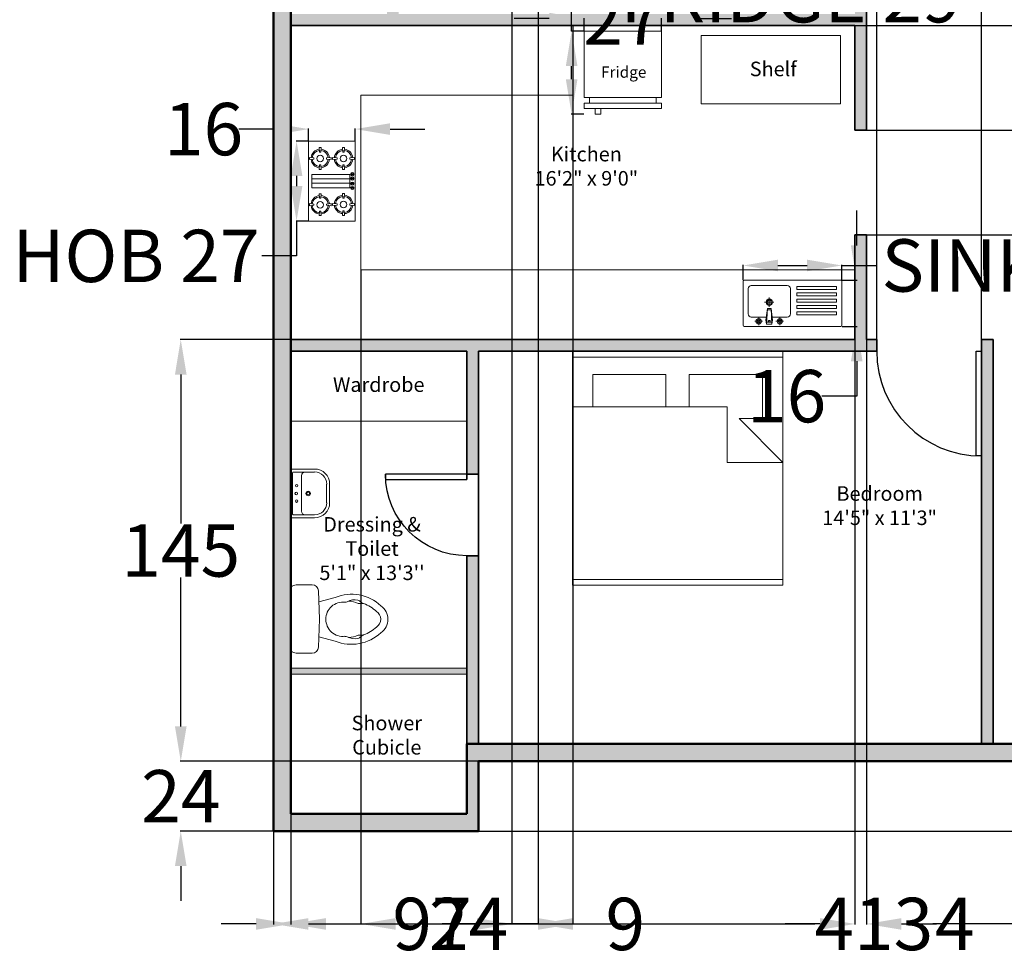
# Model space of a CAD drawing. Units: inches. Extents: x 2 to 695, y -374 to 352.
# Tile 1 of 6: x 59 to 398, y -374 to -51. Entities that reach past the tile are written whole.
import ezdxf

# ---------------------------------------------------------------- set-up
doc = ezdxf.new("R2010")
doc.units = ezdxf.units.IN
for name, color, linetype, lineweight in [('A-ANNO-DIMS', 2, 'Continuous', 18), ('A-ANNO-TEXT', 7, 'Continuous', 18), ('A-AREA-IDEN', 7, 'Continuous', 18), ('A-DOOR', 3, 'Continuous', 25), ('A-FLOR-FIXT', 9, 'Continuous', 18), ('A-WALL-PATT', 252, 'Continuous', 13), ('Furniture', 2, 'Continuous', 18), ('Inner Wall', 5, 'Continuous', 35), ('Kitchen', 6, 'Continuous', 18), ('Outer Wall', 1, 'Continuous', 50)]:
    doc.layers.add(name, color=color, linetype=linetype, lineweight=lineweight)
doc.styles.get("Standard").update_dxf_attribs({"font": 'arial.ttf'})
doc.dimstyles.get("Standard").update_dxf_attribs({"dimtxt": 18, "dimasz": 12, "dimexe": 0.18, "dimexo": 0.0625, "dimgap": 0.09, "dimtad": 0, "dimtih": 1, "dimtoh": 1, "dimdec": 0, "dimzin": 0, "dimdsep": 46, "dimlunit": 3, "dimtxsty": 'Standard', "dimcen": 0.09, "dimadec": 0, "dimazin": 0, "dimtfac": 1, "dimtdec": 0, "dimtofl": 0, "dimtmove": 0, "dimatfit": 3, "dimfxl": 1, "dimtolj": 1, "dimtzin": 0, "dimarcsym": 0})

# ---------------------------------------------------------------- blocks, each defined once
blk = doc.blocks.new('*U2')
for p, q in [((0, 0), (0, -4)), ((36, 0), (36, -4))]:
    blk.add_line(p, q)
blk.add_lwpolyline([(0, 0), (0, 36), (1.75, 36), (1.75, 0)], close=True)
blk.add_arc((0, 0), 36, 0, 90)
blk = doc.blocks.new('A$C7C492201')
for p, q in [((0, 10), (0, 426.6)), ((10, 436.6), (927.3, 436.6)), ((111.9, 388.7), (185, 388.7)), ((148.5, 425.2), (148.5, 352.2)), ((223.5, 415), (217, 376.2)), ((217, 376.2), (231.8, 268.5)), ((223.5, 415), (231.8, 268.5)), ((223.5, 415), (248.5, 415)), ((224.6, 395.4), (248.5, 395.4)), ((273.5, 415), (248.5, 415)), ((272.3, 395.4), (248.5, 395.4)), ((273.5, 415), (265.2, 268.5)), ((279.9, 376.2), (265.2, 268.5)), ((273.5, 415), (279.9, 376.2)), ((311.9, 388.7), (385, 388.7)), ((348.5, 425.2), (348.5, 352.2)), ((937.3, 10), (937.3, 426.6)), ((48.5, 318.8), (48.5, 78.8)), ((220.8, 348.8), (78.5, 348.8)), ((418.5, 348.8), (276.2, 348.8)), ((448.5, 318.8), (448.5, 78.8)), ((509.1, 328.4), (509.1, 298.4)), ((509.1, 328.4), (885, 328.4)), ((509.1, 298.4), (885, 298.4)), ((885, 328.4), (885, 298.4)), ((203.4, 207.7), (293.5, 207.7)), ((231.3, 278.6), (248.5, 278.6)), ((231.8, 268.5), (248.5, 268.5)), ((265.6, 278.6), (248.5, 278.6)), ((265.2, 268.5), (248.5, 268.5)), ((248.5, 252.8), (248.5, 162.6)), ((509.1, 268.4), (509.1, 238.4)), ((509.1, 268.4), (885, 268.4)), ((509.1, 238.4), (885, 238.4)), ((509.1, 208.4), (885, 208.4)), ((509.1, 208.4), (509.1, 178.4)), ((885, 268.4), (885, 238.4)), ((885, 208.4), (885, 178.4)), ((509.1, 178.4), (885, 178.4)), ((509.1, 148.4), (509.1, 118.4)), ((509.1, 148.4), (885, 148.4)), ((509.1, 118.4), (885, 118.4)), ((885, 148.4), (885, 118.4)), ((927.3, 0), (10, 0)), ((418.5, 48.8), (78.5, 48.8)), ((509.1, 88.4), (509.1, 58.4)), ((509.1, 88.4), (885, 88.4)), ((509.1, 58.4), (885, 58.4)), ((885, 88.4), (885, 58.4))]:
    blk.add_line(p, q)
for centre, radius in [((148.5, 388.7), 25), ((148.5, 388.7), 15), ((348.5, 388.7), 25), ((348.5, 388.7), 15), ((248.5, 207.7), 30), ((248.5, 207.7), 20)]:
    blk.add_circle(centre, radius)
for centre, radius, start, end in [((10, 426.6), 10, 90, 180), ((247.3, 388), 7.19, 80.52523, 279.47477), ((249.6, 388), 7.19, 260.52523, 99.47477), ((927.3, 426.6), 10, 0, 90), ((78.5, 318.8), 30, 90, 180), ((418.5, 318.8), 30, 0, 90), ((10, 10), 10, 180, 270), ((78.5, 78.8), 30, 180, 270), ((418.5, 78.8), 30, 270, 0), ((927.3, 10), 10, 270, 0)]:
    blk.add_arc(centre, radius, start, end)
blk = doc.blocks.new('A$C57CF26DA')
for p, q in [((0, 0), (0, 420)), ((720, 420), (0, 420)), ((166.9, 413), (146.9, 413)), ((146.9, 413), (151.9, 373)), ((151.9, 373), (161.9, 373)), ((161.9, 373), (166.9, 413)), ((300, 390.9), (300, 49.1)), ((300, 390.9), (420, 390.9)), ((340, 390.9), (340, 49.1)), ((380, 390.9), (380, 49.1)), ((420, 390.9), (420, 49.1)), ((583.6, 413), (563.6, 413)), ((563.6, 413), (568.6, 373)), ((568.6, 373), (578.6, 373)), ((578.6, 373), (583.6, 413)), ((720, 0), (720, 420)), ((98.9, 320), (58.9, 325)), ((58.9, 325), (58.9, 305)), ((58.9, 305), (98.9, 310)), ((98.9, 310), (98.9, 320)), ((254.8, 325), (214.8, 320)), ((214.8, 320), (214.8, 310)), ((214.8, 310), (254.8, 305)), ((254.8, 305), (254.8, 325)), ((515.6, 320), (475.6, 325)), ((475.6, 325), (475.6, 305)), ((475.6, 305), (515.6, 310)), ((515.6, 310), (515.6, 320)), ((671.6, 325), (631.6, 320)), ((631.6, 320), (631.6, 310)), ((631.6, 310), (671.6, 305)), ((671.6, 305), (671.6, 325)), ((151.9, 257), (146.9, 217)), ((146.9, 217), (166.9, 217)), ((166.9, 203), (146.9, 203)), ((146.9, 203), (151.9, 163)), ((161.9, 257), (151.9, 257)), ((166.9, 217), (161.9, 257)), ((161.9, 163), (166.9, 203)), ((581.1, 203), (561.1, 203)), ((561.1, 203), (566.1, 163)), ((568.6, 257), (563.6, 217)), ((563.6, 217), (583.6, 217)), ((578.6, 257), (568.6, 257)), ((576.1, 163), (581.1, 203)), ((583.6, 217), (578.6, 257)), ((98.9, 110), (58.9, 115)), ((58.9, 115), (58.9, 95)), ((58.9, 95), (98.9, 100)), ((98.9, 100), (98.9, 110)), ((151.9, 163), (161.9, 163)), ((254.8, 115), (214.8, 110)), ((214.8, 110), (214.8, 100)), ((214.8, 100), (254.8, 95)), ((254.8, 95), (254.8, 115)), ((513.1, 110), (473.1, 115)), ((473.1, 115), (473.1, 95)), ((473.1, 95), (513.1, 100)), ((513.1, 100), (513.1, 110)), ((566.1, 163), (576.1, 163)), ((669, 115), (629, 110)), ((629, 110), (629, 100)), ((629, 100), (669, 95)), ((669, 95), (669, 115)), ((151.9, 47), (146.9, 7)), ((146.9, 7), (166.9, 7)), ((161.9, 47), (151.9, 47)), ((166.9, 7), (161.9, 47)), ((301.5, 38.7), (294.7, 38.7)), ((294.7, 38.7), (294.7, 11.3)), ((294.7, 11.3), (301.5, 11.3)), ((420, 49.1), (300, 49.1)), ((301.5, 11.3), (301.5, 38.7)), ((340.5, 38.7), (333.7, 38.7)), ((333.7, 38.7), (333.7, 11.3)), ((333.7, 11.3), (340.5, 11.3)), ((340.5, 11.3), (340.5, 38.7)), ((379.7, 11.3), (379.7, 38.7)), ((379.7, 38.7), (386.5, 38.7)), ((386.5, 11.3), (379.7, 11.3)), ((386.5, 38.7), (386.5, 11.3)), ((418.7, 11.3), (418.7, 38.7)), ((418.7, 38.7), (425.5, 38.7)), ((425.5, 11.3), (418.7, 11.3)), ((425.5, 38.7), (425.5, 11.3)), ((566.1, 47), (561.1, 7)), ((561.1, 7), (581.1, 7)), ((576.1, 47), (566.1, 47)), ((581.1, 7), (576.1, 47)), ((720, 0), (0, 0))]:
    blk.add_line(p, q)
for centre in [(156.9, 315), (573.6, 315), (156.9, 105), (571.1, 105)]:
    blk.add_circle(centre, 30)
for centre, radius, start, end in [((156.9, 315), 83, 95.58493, 174.41507), ((156.9, 315), 73, 95.37384, 174.62616), ((156.9, 315), 73, 5.37384, 84.62616), ((156.9, 315), 83, 5.58493, 84.41507), ((573.6, 315), 83, 95.58493, 174.41507), ((573.6, 315), 73, 95.37384, 174.62616), ((573.6, 315), 73, 5.37384, 84.62616), ((573.6, 315), 83, 5.58493, 84.41507), ((156.9, 315), 83, 185.58493, 264.41507), ((156.9, 315), 73, 185.37384, 264.62616), ((156.9, 315), 73, 275.37384, 354.62616), ((156.9, 315), 83, 275.58493, 354.41507), ((573.6, 315), 83, 185.58493, 264.41507), ((573.6, 315), 73, 185.37384, 264.62616), ((573.6, 315), 73, 275.37384, 354.62616), ((573.6, 315), 83, 275.58493, 354.41507), ((156.9, 105), 83, 95.58493, 174.41507), ((156.9, 105), 73, 95.37384, 174.62616), ((156.9, 105), 73, 5.37384, 84.62616), ((156.9, 105), 83, 5.58493, 84.41507), ((571.1, 105), 83, 95.58493, 174.41507), ((571.1, 105), 73, 95.37384, 174.62616), ((571.1, 105), 73, 5.37384, 84.62616), ((571.1, 105), 83, 5.58493, 84.41507), ((156.9, 105), 83, 185.58493, 264.41507), ((156.9, 105), 73, 185.37384, 264.62616), ((156.9, 105), 73, 275.37384, 354.62616), ((156.9, 105), 83, 275.58493, 354.41507), ((571.1, 105), 83, 185.58493, 264.41507), ((571.1, 105), 73, 185.37384, 264.62616), ((571.1, 105), 73, 275.37384, 354.62616), ((571.1, 105), 83, 275.58493, 354.41507), ((298.1, 25), 13.7, 104.47751, 255.52249), ((298.1, 25), 13.7, 284.47751, 75.52249), ((337.1, 25), 13.7, 104.47751, 255.52249), ((337.1, 25), 13.7, 284.47751, 75.52249), ((383.1, 25), 13.7, 104.47751, 255.52249), ((383.1, 25), 13.7, 284.47751, 75.52249), ((422.1, 25), 13.7, 104.47751, 255.52249), ((422.1, 25), 13.7, 284.47751, 75.52249)]:
    blk.add_arc(centre, radius, start, end)
blk = doc.blocks.new('KING-00')
for p, q in [((-0.8967, -0.947), (-0.8967, 0.8818)), ((0.6019, 0.8818), (0.6019, -0.4644)), ((1.0337, -0.947), (1.0337, 0.8818)), ((0.6019, 0.704), (0.8813, 0.704)), ((0.8813, 0.069), (0.8813, 0.704)), ((0.6019, 0.069), (0.8813, 0.069)), ((0.8813, -0.1342), (0.6019, -0.1342)), ((0.8813, -0.7692), (0.8813, -0.1342)), ((0.1193, -0.4644), (0.1193, -0.947)), ((0.6019, -0.4644), (0.1193, -0.4644)), ((0.1193, -0.947), (0.5003, -0.566)), ((0.5003, -0.7692), (0.5003, -0.566)), ((0.5003, -0.7692), (0.8813, -0.7692))]:
    blk.add_line(p, q)
blk.add_lwpolyline([(-0.9475, -0.947), (-0.9475, 0.8818), (1.0845, 0.8818), (1.0845, -0.947)], close=True)
blk = doc.blocks.new('REFRI-00')
for points in [[(-0.35, 0.35), (-0.35, -0.25), (0.35, -0.25), (0.35, 0.35), (-0.35, 0.35)], [(-0.3, -0.3), (-0.3, -0.25)], [(0.3, -0.3), (0.3, -0.25)], [(-0.35, -0.3), (-0.35, -0.35), (0.35, -0.35), (0.35, -0.3), (-0.35, -0.3)], [(-0.25, -0.35), (-0.25, -0.4), (-0.2, -0.4), (-0.2, -0.35)]]:
    blk.add_lwpolyline(points)
blk = doc.blocks.new('A$C1308471B')
at = {"ltscale": 20}
for p, q in [((0, 0.4607), (0, 0.0186)), ((0.0354, 0.4793), (0.1495, 0.4793)), ((0.2013, 0.2397), (0.1923, 0.4384)), ((0.1957, 0.3639), (0.3109, 0.3953)), ((0.5021, 0.3528), (0.4724, 0.3528)), ((0.4982, 0.3575), (0.4822, 0.3709)), ((0.2013, 0.2397), (0.1923, 0.0409)), ((0.1959, 0.1193), (0.3109, 0.0879)), ((0.5021, 0.1304), (0.4724, 0.1304)), ((0.4982, 0.1257), (0.4822, 0.1123)), ((0.0354, 0), (0.1495, 0))]:
    blk.add_line(p, q, dxfattribs=at)
for centre, radius, start, end in [((0.006, 0.4607), 0.006, 136.52689, 180), ((0.0354, 0.4328), 0.0465, 90, 136.52689), ((0.1495, 0.4365), 0.0429, 2.57554, 90), ((0.4248, 0.1104), 0.3068, 47.41345, 111.79241), ((0.3654, 0.2416), 0.1206, 83.35226, 180), ((0.3823, 0.3868), 0.0255, 263.35226, 298.57415), ((0.4494, 0.2636), 0.1148, 79.39683, 118.57415), ((0.405, 0.2159), 0.153, 63.50202, 90.45216), ((0.4658, 0.3513), 0.0255, 50, 79.39683), ((0.5146, 0.377), 0.0255, 230, 251.38812), ((0.5021, 0.3273), 0.0255, 70.3751, 90), ((0.4248, 0.1104), 0.2558, 46.61198, 70.3751), ((0.5654, 0.2416), 0.065, 0, 57.29738), ((0.5654, 0.2416), 0.116, 0, 54.71147), ((0.3654, 0.2416), 0.1206, 180, 276.64774), ((0.5654, 0.2416), 0.065, 302.70262, 0), ((0.5654, 0.2416), 0.116, 305.28853, 0), ((0.4248, 0.3728), 0.3068, 248.20759, 312.58655), ((0.4248, 0.3728), 0.2558, 289.6249, 313.38802), ((0.3823, 0.0964), 0.0255, 61.42585, 96.64774), ((0.4494, 0.2196), 0.1148, 241.42585, 280.60317), ((0.405, 0.2673), 0.153, 269.54784, 296.49798), ((0.4658, 0.1319), 0.0255, 280.60317, 310), ((0.5146, 0.1062), 0.0255, 108.61188, 130), ((0.5021, 0.1559), 0.0255, 270, 289.6249), ((0.006, 0.0186), 0.006, 180, 223.47311), ((0.0354, 0.0465), 0.0465, 223.47311, 270), ((0.1495, 0.0429), 0.0429, 270, 357.42446)]:
    blk.add_arc(centre, radius, start, end, dxfattribs=at)
blk = doc.blocks.new('A$C57EA129C')
for p, q in [((0, 0.443), (0, 0.178)), ((0.016, 0.459), (0.563, 0.459)), ((0.036, 0.432), (0.036, 0.29)), ((0.045, 0.441), (0.535, 0.441)), ((0.544, 0.432), (0.544, 0.29)), ((0.579, 0.443), (0.579, 0.178)), ((0.036, 0.29), (0.036, 0.178)), ((0.08, 0.334), (0.499, 0.334)), ((0.544, 0.29), (0.544, 0.178)), ((0.178, 0.036), (0.401, 0.036)), ((0.178, 0), (0.401, 0))]:
    blk.add_line(p, q)
for centre, radius in [((0.198, 0.392), 0.0143), ((0.29, 0.396), 0.0156), ((0.381, 0.392), 0.0143), ((0.29, 0.255), 0.0267), ((0.29, 0.255), 0.0178)]:
    blk.add_circle(centre, radius)
for centre, radius, start, end in [((0.016, 0.443), 0.016, 90, 180), ((0.045, 0.432), 0.00891, 90, 180), ((0.535, 0.432), 0.00891, 0, 90), ((0.563, 0.443), 0.016, 0, 90), ((0.08, 0.29), 0.0445, 90, 180), ((0.499, 0.29), 0.0445, 0, 90), ((0.178, 0.178), 0.178, 180, 270), ((0.178, 0.178), 0.143, 180, 270), ((0.401, 0.178), 0.178, 270, 0), ((0.401, 0.178), 0.143, 270, 0)]:
    blk.add_arc(centre, radius, start, end)
blk = doc.blocks.new('*U3')
for p, q in [((0, 0), (0, -4)), ((28, 0), (28, -4))]:
    blk.add_line(p, q)
blk.add_lwpolyline([(0, 0), (0, 28), (1.75, 28), (1.75, 0)], close=True)
blk.add_arc((0, 0), 28, 0, 90)
blk = doc.blocks.new('*D22')
at = {"layer": 'A-ANNO-DIMS', "color": 0, "lineweight": -2, "transparency": 16777216}
for p, q in [((308.29, -140.37), (308.29, -135.15)), ((320.29, -135.33), (330.3, -135.33)), ((342.3, -140.37), (342.3, -135.15)), ((342.3, -135.33), (354.3, -135.33))]:
    blk.add_line(p, q, dxfattribs=at)
at = {"layer": 'A-ANNO-DIMS', "color": 0, "transparency": 16777216}
for points in [[(320.29, -133.33), (320.29, -137.33), (308.29, -135.33)], [(330.3, -133.33), (330.3, -137.33), (342.3, -135.33)]]:
    blk.add_solid(points, dxfattribs=at)
at = {"layer": 'Defpoints', "color": 0, "transparency": 16777216}
for p in [(342.3, -135.33), (308.29, -140.43), (342.3, -140.43)]:
    blk.add_point(p, dxfattribs=at)
at = {"layer": 'A-ANNO-DIMS', "color": 0, "transparency": 16777216, "insert": (400.04, -135.33), "char_height": 18, "attachment_point": 5}
blk.add_mtext('\\A1;SINK 34', dxfattribs=at)
blk = doc.blocks.new('*D23')
at = {"layer": 'A-ANNO-DIMS', "color": 0, "lineweight": -2, "transparency": 16777216}
for p, q in [((347.4, -128.43), (347.4, -116.43)), ((342.37, -140.43), (347.58, -140.43)), ((342.37, -156.27), (347.58, -156.27)), ((347.4, -168.27), (347.4, -180.27)), ((347.4, -180.27), (335.4, -180.27))]:
    blk.add_line(p, q, dxfattribs=at)
at = {"layer": 'A-ANNO-DIMS', "color": 0, "transparency": 16777216}
for points in [[(345.4, -128.43), (349.4, -128.43), (347.4, -140.43)], [(345.4, -168.27), (349.4, -168.27), (347.4, -156.27)]]:
    blk.add_solid(points, dxfattribs=at)
at = {"layer": 'Defpoints', "color": 0, "transparency": 16777216}
for p in [(342.3, -140.43), (342.3, -156.27), (347.4, -156.27)]:
    blk.add_point(p, dxfattribs=at)
at = {"layer": 'A-ANNO-DIMS', "color": 0, "transparency": 16777216, "insert": (323.28, -180.27), "char_height": 18, "attachment_point": 5}
blk.add_mtext('\\A1;16', dxfattribs=at)
blk = doc.blocks.new('*D24')
at = {"layer": 'A-ANNO-DIMS', "color": 0, "lineweight": -2, "transparency": 16777216}
for p, q in [((158.77, -92.56), (154.53, -92.56)), ((154.71, -104.56), (154.71, -108.04)), ((158.77, -120.04), (154.53, -120.04)), ((154.71, -120.04), (154.71, -132.04)), ((154.71, -132.04), (142.71, -132.04))]:
    blk.add_line(p, q, dxfattribs=at)
at = {"layer": 'A-ANNO-DIMS', "color": 0, "transparency": 16777216}
for points in [[(152.71, -104.56), (156.71, -104.56), (154.71, -92.56)], [(152.71, -108.04), (156.71, -108.04), (154.71, -120.04)]]:
    blk.add_solid(points, dxfattribs=at)
at = {"layer": 'Defpoints', "color": 0, "transparency": 16777216}
for p in [(158.84, -92.56), (154.71, -120.04), (158.84, -120.04)]:
    blk.add_point(p, dxfattribs=at)
at = {"layer": 'A-ANNO-DIMS', "color": 0, "transparency": 16777216, "insert": (99.48, -132.04), "char_height": 18, "attachment_point": 5}
blk.add_mtext('\\A1;HOB 27', dxfattribs=at)
blk = doc.blocks.new('*D25')
at = {"layer": 'A-ANNO-DIMS', "color": 0, "lineweight": -2, "transparency": 16777216}
for p, q in [((146.84, -88.44), (134.84, -88.44)), ((158.84, -92.5), (158.84, -88.26)), ((174.87, -92.5), (174.87, -88.26)), ((186.87, -88.44), (198.87, -88.44))]:
    blk.add_line(p, q, dxfattribs=at)
at = {"layer": 'A-ANNO-DIMS', "color": 0, "transparency": 16777216}
for points in [[(146.84, -86.44), (146.84, -90.44), (158.84, -88.44)], [(186.87, -86.44), (186.87, -90.44), (174.87, -88.44)]]:
    blk.add_solid(points, dxfattribs=at)
at = {"layer": 'Defpoints', "color": 0, "transparency": 16777216}
for p in [(158.84, -88.44), (158.84, -92.56), (174.87, -92.56)]:
    blk.add_point(p, dxfattribs=at)
at = {"layer": 'A-ANNO-DIMS', "color": 0, "transparency": 16777216, "insert": (122.71, -88.44), "char_height": 18, "attachment_point": 5}
blk.add_mtext('\\A1;16', dxfattribs=at)
blk = doc.blocks.new('*D26')
at = {"layer": 'A-ANNO-DIMS', "color": 0, "lineweight": -2, "transparency": 16777216}
for p, q in [((249.33, -54.75), (249.33, -42.75)), ((249.33, -42.75), (261.33, -42.75)), ((253.55, -54.75), (249.15, -54.75)), ((249.33, -71.32), (249.33, -66.75)), ((253.55, -83.32), (249.15, -83.32))]:
    blk.add_line(p, q, dxfattribs=at)
at = {"layer": 'A-ANNO-DIMS', "color": 0, "transparency": 16777216}
for points in [[(247.33, -66.75), (251.33, -66.75), (249.33, -54.75)], [(247.33, -71.32), (251.33, -71.32), (249.33, -83.32)]]:
    blk.add_solid(points, dxfattribs=at)
at = {"layer": 'Defpoints', "color": 0, "transparency": 16777216}
for p in [(249.33, -54.75), (253.61, -54.75), (253.61, -83.32)]:
    blk.add_point(p, dxfattribs=at)
at = {"layer": 'A-ANNO-DIMS', "color": 0, "transparency": 16777216, "insert": (324.81, -42.75), "char_height": 18, "attachment_point": 5}
blk.add_mtext('\\A1;FRIDGE 29', dxfattribs=at)
blk = doc.blocks.new('*D27')
at = {"layer": 'A-ANNO-DIMS', "color": 0, "lineweight": -2, "transparency": 16777216}
for p, q in [((241.61, -50.46), (229.61, -50.46)), ((253.61, -54.69), (253.61, -50.28)), ((280.28, -54.69), (280.28, -50.28)), ((292.28, -50.46), (304.28, -50.46))]:
    blk.add_line(p, q, dxfattribs=at)
at = {"layer": 'A-ANNO-DIMS', "color": 0, "transparency": 16777216}
for points in [[(241.61, -48.46), (241.61, -52.46), (253.61, -50.46)], [(292.28, -48.46), (292.28, -52.46), (280.28, -50.46)]]:
    blk.add_solid(points, dxfattribs=at)
at = {"layer": 'Defpoints', "color": 0, "transparency": 16777216}
for p in [(280.28, -50.46), (253.61, -54.75), (280.28, -54.75)]:
    blk.add_point(p, dxfattribs=at)
at = {"layer": 'A-ANNO-DIMS', "color": 0, "transparency": 16777216, "insert": (266.94, -50.46), "char_height": 18, "attachment_point": 5}
blk.add_mtext('\\A1;27', dxfattribs=at)
blk = doc.blocks.new('*D28')
at = {"layer": 'A-ANNO-DIMS', "color": 0, "lineweight": -2, "transparency": 16777216}
for p, q in [((559.79, -305.89), (559.79, -361.92)), ((146.79, -329.89), (146.79, -361.92)), ((158.79, -361.74), (332.95, -361.74)), ((547.79, -361.74), (373.62, -361.74))]:
    blk.add_line(p, q, dxfattribs=at)
at = {"layer": 'A-ANNO-DIMS', "color": 0, "transparency": 16777216}
for points in [[(158.79, -359.74), (158.79, -363.74), (146.79, -361.74)], [(547.79, -359.74), (547.79, -363.74), (559.79, -361.74)]]:
    blk.add_solid(points, dxfattribs=at)
at = {"layer": 'Defpoints', "color": 0, "transparency": 16777216}
for p in [(559.79, -305.82), (146.79, -329.82), (559.79, -361.74)]:
    blk.add_point(p, dxfattribs=at)
at = {"layer": 'A-ANNO-DIMS', "color": 0, "transparency": 16777216, "insert": (353.29, -361.74), "char_height": 18, "attachment_point": 5}
blk.add_mtext('\\A1;413', dxfattribs=at)
blk = doc.blocks.new('*D29')
at = {"layer": 'A-ANNO-DIMS', "color": 0, "lineweight": -2, "transparency": 16777216}
for p, q in [((420.85, 308.13), (591.88, 308.13)), ((591.7, 296.13), (591.7, -1.56)), ((591.7, -317.82), (591.7, -20.13)), ((217.35, -329.82), (591.88, -329.82))]:
    blk.add_line(p, q, dxfattribs=at)
at = {"layer": 'A-ANNO-DIMS', "color": 0, "transparency": 16777216}
for points in [[(589.7, 296.13), (593.7, 296.13), (591.7, 308.13)], [(589.7, -317.82), (593.7, -317.82), (591.7, -329.82)]]:
    blk.add_solid(points, dxfattribs=at)
at = {"layer": 'Defpoints', "color": 0, "transparency": 16777216}
for p in [(420.79, 308.13), (591.7, 308.13), (217.29, -329.82)]:
    blk.add_point(p, dxfattribs=at)
at = {"layer": 'A-ANNO-DIMS', "color": 0, "transparency": 16777216, "insert": (591.7, -10.85), "char_height": 18, "attachment_point": 5}
blk.add_mtext('\\A1;638', dxfattribs=at)
blk = doc.blocks.new('*D35')
at = {"layer": 'A-ANNO-DIMS', "color": 0, "lineweight": -2, "transparency": 16777216}
for p, q in [((114.870845, -293.824954), (114.870845, -281.824954)), ((217.223345, -305.824954), (114.690845, -305.824954)), ((146.723345, -329.824954), (114.690845, -329.824954)), ((114.870845, -341.824954), (114.870845, -353.824954))]:
    blk.add_line(p, q, dxfattribs=at)
at = {"layer": 'A-ANNO-DIMS', "color": 0, "transparency": 16777216}
for points in [[(112.870845, -293.824954), (116.870845, -293.824954), (114.870845, -305.824954)], [(112.870845, -341.824954), (116.870845, -341.824954), (114.870845, -329.824954)]]:
    blk.add_solid(points, dxfattribs=at)
at = {"layer": 'Defpoints', "color": 0, "transparency": 16777216}
for p in [(114.870845, -305.824954), (217.285845, -305.824954), (146.785845, -329.824954)]:
    blk.add_point(p, dxfattribs=at)
at = {"layer": 'A-ANNO-DIMS', "color": 0, "transparency": 16777216, "insert": (114.870845, -317.824954), "char_height": 18, "attachment_point": 5}
blk.add_mtext('\\A1;24', dxfattribs=at)
blk = doc.blocks.new('*D36')
at = {"layer": 'A-ANNO-DIMS', "color": 0, "lineweight": -2, "transparency": 16777216}
for p, q in [((152.72, -160.82), (114.69, -160.82)), ((114.87, -172.82), (114.87, -224.04)), ((114.87, -293.82), (114.87, -242.61)), ((217.22, -305.82), (114.69, -305.82))]:
    blk.add_line(p, q, dxfattribs=at)
at = {"layer": 'A-ANNO-DIMS', "color": 0, "transparency": 16777216}
for points in [[(112.87, -172.82), (116.87, -172.82), (114.87, -160.82)], [(112.87, -293.82), (116.87, -293.82), (114.87, -305.82)]]:
    blk.add_solid(points, dxfattribs=at)
at = {"layer": 'Defpoints', "color": 0, "transparency": 16777216}
for p in [(114.87, -160.82), (152.79, -160.82), (217.29, -305.82)]:
    blk.add_point(p, dxfattribs=at)
at = {"layer": 'A-ANNO-DIMS', "color": 0, "transparency": 16777216, "insert": (114.87, -233.32), "char_height": 18, "attachment_point": 5}
blk.add_mtext('\\A1;145', dxfattribs=at)
blk = doc.blocks.new('*D37')
at = {"layer": 'A-ANNO-DIMS', "color": 0, "lineweight": -2, "transparency": 16777216}
for p, q in [((350.85, -88.82), (591.88, -88.82)), ((591.7, -100.82), (591.7, -112.82)), ((350.85, -124.82), (591.88, -124.82)), ((591.7, -124.82), (591.7, -136.82)), ((591.7, -136.82), (579.7, -136.82))]:
    blk.add_line(p, q, dxfattribs=at)
at = {"layer": 'A-ANNO-DIMS', "color": 0, "transparency": 16777216}
for points in [[(589.7, -100.82), (593.7, -100.82), (591.7, -88.82)], [(589.7, -112.82), (593.7, -112.82), (591.7, -124.82)]]:
    blk.add_solid(points, dxfattribs=at)
at = {"layer": 'Defpoints', "color": 0, "transparency": 16777216}
for p in [(350.79, -88.82), (350.79, -124.82), (591.7, -124.82)]:
    blk.add_point(p, dxfattribs=at)
at = {"layer": 'A-ANNO-DIMS', "color": 0, "transparency": 16777216, "insert": (566.73, -136.82), "char_height": 18, "attachment_point": 5}
blk.add_mtext('\\A1;36', dxfattribs=at)
blk = doc.blocks.new('*D41')
at = {"layer": 'A-ANNO-DIMS', "color": 0, "lineweight": -2, "transparency": 16777216}
for p, q in [((342.285845, 340.044756), (330.285845, 340.044756)), ((354.285845, -164.762454), (354.285845, 340.224756)), ((390.285845, -164.762454), (390.285845, 340.224756)), ((402.285845, 340.044756), (414.285845, 340.044756))]:
    blk.add_line(p, q, dxfattribs=at)
at = {"layer": 'A-ANNO-DIMS', "color": 0, "transparency": 16777216}
for points in [[(342.285845, 342.044756), (342.285845, 338.044756), (354.285845, 340.044756)], [(402.285845, 342.044756), (402.285845, 338.044756), (390.285845, 340.044756)]]:
    blk.add_solid(points, dxfattribs=at)
at = {"layer": 'Defpoints', "color": 0, "transparency": 16777216}
for p in [(390.285845, 340.044756), (354.285845, -164.824954), (390.285845, -164.824954)]:
    blk.add_point(p, dxfattribs=at)
at = {"layer": 'A-ANNO-DIMS', "color": 0, "transparency": 16777216, "insert": (372.285845, 340.044756), "char_height": 18, "attachment_point": 5}
blk.add_mtext('\\A1;36', dxfattribs=at)
blk = doc.blocks.new('*D42')
at = {"layer": 'A-ANNO-DIMS', "color": 0, "lineweight": -2, "transparency": 16777216}
for p, q in [((176.79, -136.89), (176.79, -361.92)), ((152.79, -160.89), (152.79, -361.92)), ((140.79, -361.74), (128.79, -361.74)), ((188.79, -361.74), (200.79, -361.74))]:
    blk.add_line(p, q, dxfattribs=at)
at = {"layer": 'A-ANNO-DIMS', "color": 0, "transparency": 16777216}
for points in [[(140.79, -359.74), (140.79, -363.74), (152.79, -361.74)], [(188.79, -359.74), (188.79, -363.74), (176.79, -361.74)]]:
    blk.add_solid(points, dxfattribs=at)
at = {"layer": 'Defpoints', "color": 0, "transparency": 16777216}
for p in [(176.79, -136.82), (152.79, -160.82), (176.79, -361.74)]:
    blk.add_point(p, dxfattribs=at)
at = {"layer": 'A-ANNO-DIMS', "color": 0, "transparency": 16777216, "insert": (213.88, -361.74), "char_height": 18, "attachment_point": 5}
blk.add_mtext('\\A1;24', dxfattribs=at)
blk = doc.blocks.new('*D43')
at = {"layer": 'A-ANNO-DIMS', "color": 0, "lineweight": -2, "transparency": 16777216}
for p, q in [((152.79, -52.89), (152.79, -361.92)), ((249.79, -52.89), (249.79, -361.92)), ((164.79, -361.74), (188.3, -361.74)), ((237.79, -361.74), (214.27, -361.74))]:
    blk.add_line(p, q, dxfattribs=at)
at = {"layer": 'A-ANNO-DIMS', "color": 0, "transparency": 16777216}
for points in [[(164.79, -359.74), (164.79, -363.74), (152.79, -361.74)], [(237.79, -359.74), (237.79, -363.74), (249.79, -361.74)]]:
    blk.add_solid(points, dxfattribs=at)
at = {"layer": 'Defpoints', "color": 0, "transparency": 16777216}
for p in [(152.79, -52.82), (249.79, -52.82), (249.79, -361.74)]:
    blk.add_point(p, dxfattribs=at)
at = {"layer": 'A-ANNO-DIMS', "color": 0, "transparency": 16777216, "insert": (201.29, -361.74), "char_height": 18, "attachment_point": 5}
blk.add_mtext('\\A1;97', dxfattribs=at)
blk = doc.blocks.new('*D44')
at = {"layer": 'A-ANNO-DIMS', "color": 0, "lineweight": -2, "transparency": 16777216}
for p, q in [((346.79, -160.89), (346.79, -361.92)), ((350.79, -160.89), (350.79, -361.92)), ((334.79, -361.74), (322.79, -361.74)), ((362.79, -361.74), (374.79, -361.74))]:
    blk.add_line(p, q, dxfattribs=at)
at = {"layer": 'A-ANNO-DIMS', "color": 0, "transparency": 16777216}
for points in [[(334.79, -359.74), (334.79, -363.74), (346.79, -361.74)], [(362.79, -359.74), (362.79, -363.74), (350.79, -361.74)]]:
    blk.add_solid(points, dxfattribs=at)
at = {"layer": 'Defpoints', "color": 0, "transparency": 16777216}
for p in [(346.79, -160.82), (350.79, -160.82), (350.79, -361.74)]:
    blk.add_point(p, dxfattribs=at)
at = {"layer": 'A-ANNO-DIMS', "color": 0, "transparency": 16777216, "insert": (381.1, -361.74), "char_height": 18, "attachment_point": 5}
blk.add_mtext('\\A1;4', dxfattribs=at)
blk = doc.blocks.new('*D48')
at = {"layer": 'A-ANNO-DIMS', "color": 0, "lineweight": -2, "transparency": 16777216}
for p, q in [((228.79, -9.89), (228.79, -361.92)), ((237.79, -9.89), (237.79, -361.92)), ((216.79, -361.74), (204.79, -361.74)), ((249.79, -361.74), (261.79, -361.74))]:
    blk.add_line(p, q, dxfattribs=at)
at = {"layer": 'A-ANNO-DIMS', "color": 0, "transparency": 16777216}
for points in [[(216.79, -359.74), (216.79, -363.74), (228.79, -361.74)], [(249.79, -359.74), (249.79, -363.74), (237.79, -361.74)]]:
    blk.add_solid(points, dxfattribs=at)
at = {"layer": 'Defpoints', "color": 0, "transparency": 16777216}
for p in [(228.79, -9.82), (237.79, -9.82), (237.79, -361.74)]:
    blk.add_point(p, dxfattribs=at)
at = {"layer": 'A-ANNO-DIMS', "color": 0, "transparency": 16777216, "insert": (267.79, -361.74), "char_height": 18, "attachment_point": 5}
blk.add_mtext('\\A1;9', dxfattribs=at)
blk = doc.blocks.new('*D51')
at = {"layer": 'A-ANNO-DIMS', "color": 0, "lineweight": -2, "transparency": 16777216}
for p, q in [((346.85, -52.82), (591.88, -52.82)), ((591.7, -64.82), (591.7, -76.82)), ((346.85, -88.82), (591.88, -88.82)), ((591.7, -88.82), (591.7, -100.82)), ((591.7, -100.82), (579.7, -100.82))]:
    blk.add_line(p, q, dxfattribs=at)
at = {"layer": 'A-ANNO-DIMS', "color": 0, "transparency": 16777216}
for points in [[(589.7, -64.82), (593.7, -64.82), (591.7, -52.82)], [(589.7, -76.82), (593.7, -76.82), (591.7, -88.82)]]:
    blk.add_solid(points, dxfattribs=at)
at = {"layer": 'Defpoints', "color": 0, "transparency": 16777216}
for p in [(346.79, -52.82), (346.79, -88.82), (591.7, -88.82)]:
    blk.add_point(p, dxfattribs=at)
at = {"layer": 'A-ANNO-DIMS', "color": 0, "transparency": 16777216, "insert": (566.73, -100.82), "char_height": 18, "attachment_point": 5}
blk.add_mtext('\\A1;36', dxfattribs=at)

msp = doc.modelspace()

# ---------------------------------------------------------------- hatches: boundary and pattern name
at = {"layer": 'A-WALL-PATT'}
h = msp.add_hatch(color=256, dxfattribs=at)
h.dxf.hatch_style = 1
h.paths.add_polyline_path([(346.7858, 296.175), (146.7858, 296.175), (146.7858, -329.825), (217.2858, -329.825), (217.2858, -305.825), (559.7858, -305.825), (559.7858, 296.175), (420.7858, 296.175), (420.7858, 290.175), (553.7858, 290.175), (553.7858, -299.825), (213.2858, -299.825), (213.2858, -323.825), (152.7858, -323.825), (152.7858, 290.175), (346.7858, 290.175)])
h.paths.add_polyline_path([(420.7858, 308.1298), (346.7858, 308.1298), (346.7858, 242.175), (228.7858, 242.175), (228.7858, 264.175), (152.7858, 264.175), (152.7858, 260.175), (224.7858, 260.175), (224.7858, 236.175), (350.7858, 236.175), (350.7858, 302.1298), (416.7858, 302.1298), (416.7858, 236.175), (553.7858, 236.175), (553.7858, 242.175), (420.7858, 242.175)])
h = msp.add_hatch(color=256, dxfattribs=at)
h.dxf.hatch_style = 1
h.paths.add_polyline_path([(394.2858, -160.825), (390.2858, -160.825), (390.2858, -164.825), (390.2858, -299.825), (394.2858, -299.825)])
h.paths.add_polyline_path([(217.2858, -235.1253), (213.2858, -235.1253), (213.2858, -299.825), (217.2858, -299.825)])
h.paths.add_polyline_path([(213.2858, -273.825), (152.7858, -273.825), (152.7858, -275.825), (213.2858, -275.825)])
h.paths.add_polyline_path([(354.2858, -160.825), (350.7858, -160.825), (350.7858, -124.825), (346.7858, -124.825), (346.7858, -160.825), (152.7858, -160.825), (152.7858, -164.825), (213.2858, -164.825), (213.2858, -188.8137), (213.2858, -207.1253), (217.2858, -207.1253), (217.2858, -187.1253), (217.2858, -164.825), (354.2858, -164.825)])
h.paths.add_polyline_path([(350.7858, -20.825), (346.7858, -20.825), (346.7858, -48.825), (152.7858, -48.825), (152.7858, -52.825), (249.7858, -52.825), (346.7858, -52.825), (346.7858, -88.825), (350.7858, -88.825)])
h.paths.add_polyline_path([(189.7858, 33.175), (185.7858, 33.175), (185.7858, -48.825), (189.7858, -48.825)])
h.paths.add_polyline_path([(334.7858, 37.175), (264.7858, 37.175), (264.7858, 33.175), (334.7858, 33.175)])
h.paths.add_polyline_path([(258.7858, 37.175), (152.7858, 37.175), (152.7858, 33.175), (258.7858, 33.175)])
h.paths.add_polyline_path([(194.7858, 101.175), (192.7858, 101.175), (192.7858, 37.175), (194.7858, 37.175)])
h.paths.add_polyline_path([(264.7858, 105.175), (258.7858, 105.175), (258.7858, 33.175), (264.7858, 33.175), (264.7858, 37.175)])
h.paths.add_polyline_path([(340.7858, 105.175), (334.7858, 105.175), (334.7858, 33.175), (340.7858, 33.175)])
h.paths.add_polyline_path([(350.7858, 111.175), (346.7858, 111.175), (346.7858, 105.175), (340.7858, 105.175), (340.7858, 101.175), (350.7858, 101.175)])
h.paths.add_polyline_path([(350.7858, 37.175), (340.7858, 37.175), (340.7858, 33.175), (346.7858, 33.175), (346.7858, 27.175), (350.7858, 27.175)])
h.paths.add_polyline_path([(334.7858, 105.175), (264.7858, 105.175), (264.7858, 101.175), (334.7858, 101.175)])
h.paths.add_polyline_path([(258.7858, 105.175), (252.7858, 105.175), (252.7858, 101.175), (258.7858, 101.175)])
h.paths.add_polyline_path([(224.7858, 105.175), (152.7858, 105.175), (152.7858, 101.175), (224.7858, 101.175)])
h.paths.add_polyline_path([(382.7858, 165.1298), (350.7858, 165.1298), (350.7858, 161.1298), (382.7858, 161.1298)])
h.paths.add_polyline_path([(350.7858, 236.175), (346.7858, 236.175), (346.7858, 147.175), (350.7858, 147.175)])
h.paths.add_polyline_path([(420.7858, 202.175), (416.7858, 202.175), (416.7858, 101.175), (420.7858, 101.175)])
h.paths.add_polyline_path([(416.7858, 165.1298), (410.7858, 165.1298), (410.7858, 161.1298), (416.7858, 161.1298)])
h.paths.add_polyline_path([(416.7858, 242.175), (350.7858, 242.175), (350.7858, 240.175), (416.7858, 240.175)])
h.paths.add_polyline_path([(420.7858, 236.175), (416.7858, 236.175), (416.7858, 230.175), (420.7858, 230.175)])
h.paths.add_polyline_path([(553.7858, 59.175), (469.3071, 59.175), (420.7858, 59.175), (420.7858, 65.175), (416.7858, 65.175), (416.7858, 55.175), (553.7858, 55.175)])

# ---------------------------------------------------------------- linework, layer by layer
at = {"layer": 'A-FLOR-FIXT'}
for p, q in [((213.2858, -273.825), (152.7858, -273.825)), ((213.2858, -275.825), (152.7858, -275.825))]:
    msp.add_line(p, q, dxfattribs=at)
at = {"layer": 'Furniture'}
msp.add_lwpolyline([(152.7858, -164.825), (213.2858, -164.825), (213.2858, -188.8137), (152.7858, -188.8137)], close=True, dxfattribs=at)
at = {"layer": 'Inner Wall'}
for p, q in [((350.7858, -88.825), (350.7858, -20.825)), ((346.7858, -52.825), (152.7858, -52.825)), ((346.7858, -88.825), (346.7858, -52.825)), ((346.7858, -88.825), (350.7858, -88.825)), ((346.7858, -160.825), (346.7858, -124.825)), ((346.7858, -124.825), (350.7858, -124.825)), ((350.7858, -160.825), (350.7858, -124.825)), ((346.7858, -160.825), (152.7858, -160.825)), ((354.2858, -160.825), (350.7858, -160.825)), ((354.2858, -164.825), (354.2858, -160.825)), ((394.2858, -160.825), (390.2858, -160.825)), ((390.2858, -164.825), (390.2858, -160.825)), ((394.2858, -299.825), (394.2858, -160.825)), ((213.2858, -164.825), (152.7858, -164.825)), ((213.2858, -208.8753), (213.2858, -164.825)), ((354.2858, -164.825), (217.2858, -164.825)), ((217.2858, -207.1253), (217.2858, -164.825)), ((390.2858, -299.825), (390.2858, -164.825)), ((217.2858, -235.1253), (217.2858, -187.1253)), ((213.2858, -207.1253), (217.2858, -207.1253)), ((213.2858, -299.825), (213.2858, -235.1253)), ((213.2858, -235.1253), (217.2858, -235.1253)), ((217.2858, -299.825), (217.2858, -235.1253))]:
    msp.add_line(p, q, dxfattribs=at)
at = {"layer": 'Kitchen'}
msp.add_lwpolyline([(346.7858, -136.825), (346.7858, -160.825), (152.7858, -160.825), (152.7858, -52.825), (249.7858, -52.825), (249.7858, -76.825), (176.7858, -76.825), (176.7858, -136.825), (346.7858, -136.825)], dxfattribs=at)
msp.add_lwpolyline([(293.8461, -56.2422), (341.8461, -56.2422), (341.8461, -79.7598), (293.8461, -79.7598)], close=True, dxfattribs=at)
at = {"layer": 'Outer Wall'}
for p, q in [((146.7858, -329.825), (146.7858, 296.175)), ((152.7858, -323.825), (152.7858, 290.175)), ((553.7858, -299.825), (213.2858, -299.825)), ((213.2858, -323.825), (213.2858, -299.825)), ((217.2858, -329.825), (217.2858, -305.825)), ((559.7858, -305.825), (217.2858, -305.825)), ((213.2858, -323.825), (152.7858, -323.825)), ((217.2858, -329.825), (146.7858, -329.825))]:
    msp.add_line(p, q, dxfattribs=at)

# ---------------------------------------------------------------- block references
at = {"layer": 'A-DOOR', "rotation": 180}
msp.add_blockref('*U2', (390.2858, -164.825), dxfattribs=at)
at = {"layer": 'A-DOOR', "xscale": -1, "rotation": 89.99999999999991}
msp.add_blockref('*U3', (213.2858, -207.1253), dxfattribs=at)
at = {"layer": 'A-FLOR-FIXT'}
for name, p, xscale, yscale, zscale, rotation in [('A$C57EA129C', (166.0853, -205.3193), -28.98333223671166, 28.98333223671166, 28.98333223671166, 90), ('A$C1308471B', (152.7858, -245.1543), -48.95497407897215, 48.95497407897215, 48.95497407897215, 180)]:
    msp.add_blockref(name, p, dxfattribs=dict(at, xscale=xscale, yscale=yscale, zscale=zscale, rotation=rotation))
at = {"layer": 'Furniture', "xscale": 39.60249106241186, "yscale": 39.60249106241186, "zscale": 39.60249106241186, "rotation": 89.99999999999999}
msp.add_blockref('KING-00', (284.4961, -207.7738), dxfattribs=at)
at = {"layer": 'Kitchen', "xscale": 38.0932829071003, "yscale": 38.0932829071003, "zscale": 38.0932829071003}
msp.add_blockref('REFRI-00', (266.944, -68.0814), dxfattribs=at)
at = {"layer": 'Kitchen'}
for name, p, xscale, yscale, zscale, rotation in [('A$C57CF26DA', (174.8686, -92.5605), -0.0381707681172169, 0.0381707681172169, 0.0381707681172169, 90), ('A$C7C492201', (308.2945, -140.4295), -0.0362851414289068, 0.0362851414289068, 0.0362851414289068, 180)]:
    msp.add_blockref(name, p, dxfattribs=dict(at, xscale=xscale, yscale=yscale, zscale=zscale, rotation=rotation))

# ---------------------------------------------------------------- texts
at = {"layer": 'A-ANNO-TEXT'}
for s, width, gutter_width, insert, char_height, attachment_point in [('\\pxqc;{\\fTimes New Roman|b0|i0|c0|p18;Fridge}', 17.951771, 4.8475, (258.2692, -66.8987), 3.877971, 1), ('\\pxqc;{\\fTimes New Roman|b0|i0|c0|p18;Shelf}', 49.101878, 12.5, (343.2322, -65.2576), 5, 3), ('\\pxqc;{\\fTimes New Roman|b0|i0|c0|p18;Wardrobe}', 49.101878, 12.5, (207.5173, -173.8), 5, 3), ('\\pxqc;{\\fTimes New Roman|b0|i0|c0|p18;Shower\\PCubicle}', 49.101878, 12.5, (210.3004, -290.1556), 5, 3)]:
    msp.add_mtext_dynamic_manual_height_columns(s, width=width, gutter_width=gutter_width, heights=[0], dxfattribs=dict(at, insert=insert, char_height=char_height, attachment_point=attachment_point))
at = {"layer": 'A-AREA-IDEN', "char_height": 5, "attachment_point": 3}
for s, insert in [('\\pxqc;{\\fTimes New Roman|b0|i0|c0|p18;Kitchen \\P16\'2" x 9\'0"}', (278.944, -94.5315)), ('\\pxqc;{\\fTimes New Roman|b0|i0|c0|p18;Bedroom\\P14\'5" x 11\'3"}', (379.843, -211.2464)), ('\\pxqc;{\\fTimes New Roman|b0|i0|c0|p18;Dressing & Toilet\\P5\'1" x 13\'3\'\'}', (205.2169, -221.8262))]:
    msp.add_mtext_dynamic_manual_height_columns(s, width=49.101878, gutter_width=12.5, heights=[0], dxfattribs=dict(at, insert=insert))

# ---------------------------------------------------------------- dimensions: what is measured, and where the dimension line sits
at = {"layer": 'A-ANNO-DIMS'}
for base, p1, p2, picture, middle in [((390.2858, 340.0448), (354.2858, -164.825), (390.2858, -164.825), '*D41', (372.2858, 340.0448)), ((237.7858, -361.74), (228.7858, -9.825), (237.7858, -9.825), '*D48', (267.794, -361.74)), ((280.2766, -50.4633), (253.6113, -54.7488), (280.2766, -54.7488), '*D27', (266.944, -50.4633)), ((249.7858, -361.74), (152.7858, -52.825), (249.7858, -52.825), '*D43', (201.2858, -361.74)), ((176.7858, -361.74), (152.7858, -160.825), (176.7858, -136.825), '*D42', (213.8847, -361.74)), ((350.7858, -361.74), (346.7858, -160.825), (350.7858, -160.825), '*D44', (381.1009, -361.74)), ((559.7858, -361.74), (146.7858, -329.825), (559.7858, -305.825), '*D28', (353.2858, -361.74))]:
    dim = msp.add_linear_dim(base=base, p1=p1, p2=p2, dimstyle='Standard', override={"dimdec": 0, "dimlfac": 1, "dimrnd": 0, "dimzin": 0, "dimdsep": 46, "dimlunit": 2}, dxfattribs=at)
    dim.commit()
    dim.dimension.update_dxf_attribs({"geometry": picture, "text_midpoint": middle})
for base, p1, p2, angle, picture, middle in [((591.7008, 308.1298), (217.2858, -329.825), (420.7858, 308.1298), 90, '*D29', (591.7008, -10.8476)), ((591.7008, -88.825), (346.7858, -52.825), (346.7858, -88.825), 90, '*D51', (566.7309, -100.825)), ((158.8369, -88.4381), (174.8686, -92.5605), (158.8369, -92.5605), 180, '*D25', (122.708, -88.4381)), ((591.7008, -124.825), (350.7858, -88.825), (350.7858, -124.825), 90, '*D37', (566.7309, -136.825)), ((347.4041, -156.272), (342.3028, -140.4295), (342.3028, -156.272), 270, '*D23', (323.2752, -180.272)), ((114.8708, -160.825), (217.2858, -305.825), (152.7858, -160.825), 90, '*D36', (114.8708, -233.325)), ((114.8708, -305.825), (146.7858, -329.825), (217.2858, -305.825), 90, '*D35', (114.8708, -317.825))]:
    dim = msp.add_linear_dim(base=base, p1=p1, p2=p2, angle=angle, dimstyle='Standard', override={"dimdec": 0, "dimlfac": 1, "dimrnd": 0, "dimzin": 0, "dimdsep": 46, "dimlunit": 2}, dxfattribs=at)
    dim.commit()
    dim.dimension.update_dxf_attribs({"geometry": picture, "text_midpoint": middle})
for base, p1, p2, angle, text, picture, middle in [((249.3258, -54.7488), (253.6113, -83.3188), (253.6113, -54.7488), 90, 'FRIDGE <>', '*D26', (324.8087, -42.7488)), ((154.7144, -120.0435), (158.8369, -92.5605), (158.8369, -120.0435), 270, 'HOB <>', '*D24', (99.4784, -132.0435))]:
    dim = msp.add_linear_dim(base=base, p1=p1, p2=p2, angle=angle, text=text, dimstyle='Standard', override={"dimdec": 0, "dimlfac": 1, "dimrnd": 0, "dimzin": 0, "dimdsep": 46, "dimlunit": 2}, dxfattribs=at)
    dim.commit()
    dim.dimension.update_dxf_attribs({"geometry": picture, "text_midpoint": middle})
dim = msp.add_linear_dim(base=(342.3028, -135.3283), p1=(308.2945, -140.4295), p2=(342.3028, -140.4295), text='SINK <>', dimstyle='Standard', override={"dimdec": 0, "dimlfac": 1, "dimrnd": 0, "dimzin": 0, "dimdsep": 46, "dimlunit": 2}, dxfattribs=at)
dim.commit()
dim.dimension.update_dxf_attribs({"geometry": '*D22', "text_midpoint": (400.0436, -135.3283)})

doc.saveas('drawing.dxf')
